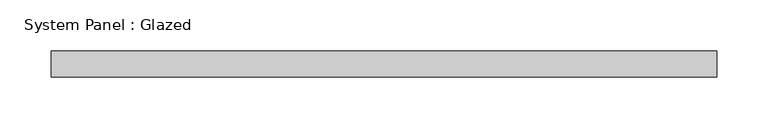
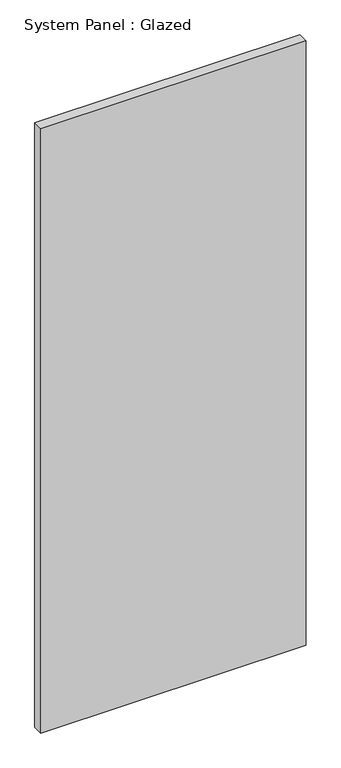
"""IFC4 building model written with IfcOpenShell, lengths in millimetres: plate geometry, System Panel : Glazed."""

from ifc_helpers import new_model, si_unit, origin, origin_with_axes, place, context, project, spatial, polyline, outline, extrude, source, transform, mapped, element, save


def system_panel_glazed_a8f3d8ee(model_context):
    return source(origin(), model_context, "Body", "SweptSolid", [
        extrude(outline(polyline([(323.85, 19.05), (-323.85, 19.05), (-323.85, 44.45), (323.85, 44.45), (323.85, 19.05)])), origin_with_axes(), (0.0, 0.0, 1.0), 1560.096911),
    ])


if __name__ == "__main__":
    model = new_model("IFC4")
    model_context = context("Model", 3, world=origin())
    ifc_project = project(units=[si_unit("LENGTHUNIT", "METRE", prefix="MILLI")], contexts=[model_context])
    site = spatial("IfcSite", under=ifc_project)
    building = spatial("IfcBuilding", under=site)
    placement = place(None, origin())
    system_panel_glazed_shape = system_panel_glazed_a8f3d8ee(model_context)
    element("IfcPlate", 1, ObjectType="System Panel : Glazed", at=placement, inside=building, context=model_context, shape_type="MappedRepresentation", body=[
        mapped(system_panel_glazed_shape, transform((0.0, 0.0, 0.0), x_axis=(1.0, 0.0, 0.0), y_axis=(0.0, 1.0, 0.0), z_axis=(0.0, 0.0, 1.0))),
    ])
    save(model, "model.ifc")

# Revit data of these elements
# Type "System Panel : Glazed"
#   Construction Type Id = "GSP4R"
#   Analytic Construction = "1/8 in Pilkington single glazing"
#   Visual Light Transmittance = 0.9
#   Solar Heat Gain Coefficient = 0.86
#   Heat Transfer Coefficient (U) = 1.18115 BTU/(h·ft²·°F)
#   Define Thermal Properties by = 1
# Element 1 (IfcPlate, "System Panel : Glazed")
#   Materials on its faces: "Glass"
# Materials
#   "Glass": class "Glass", colour RGB 0 128 192, transparency 0.75, Description = "Soda Lime Glass", Cost = 0
